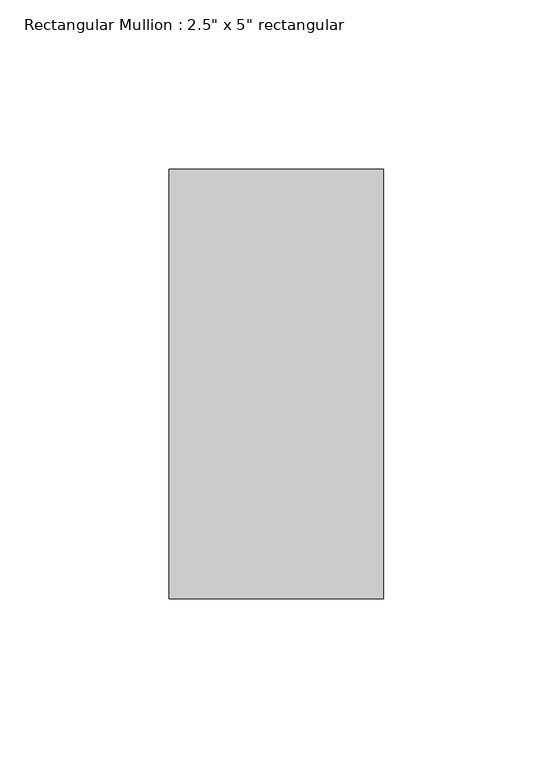
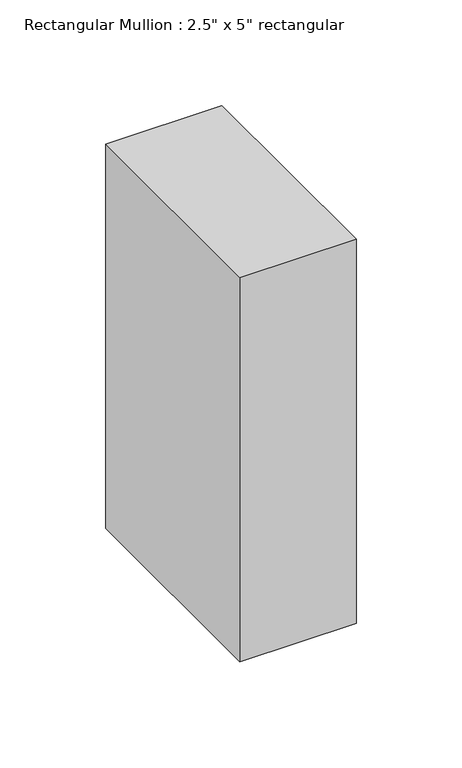
"""IFC4 building model written with IfcOpenShell, lengths in millimetres: member geometry."""

from ifc_helpers import new_model, si_unit, frame, origin, place, context, project, spatial, polyline, outline, extrude, source, transform, mapped, element, save


def member_d8da5bea(model_context):
    return source(origin(), model_context, "Body", "SweptSolid", [
        extrude(outline(polyline([(0.0, 63.5), (0.0, -63.5), (-63.5, -63.5), (-63.5, 63.5), (0.0, 63.5)])), frame((0.0, 0.0, -222.25), z_axis=(0.0, 0.0, 1.0), x_axis=(1.0, 0.0, 0.0)), (0.0, 0.0, 1.0), 222.25),
    ])


if __name__ == "__main__":
    model = new_model("IFC4")
    model_context = context("Model", 3, world=origin())
    ifc_project = project(units=[si_unit("LENGTHUNIT", "METRE", prefix="MILLI")], contexts=[model_context])
    site = spatial("IfcSite", under=ifc_project)
    building = spatial("IfcBuilding", under=site)
    placement = place(None, origin())
    member_shape = member_d8da5bea(model_context)
    element("IfcMember", 1, ObjectType="Rectangular Mullion : 2.5\" x 5\" rectangular", at=placement, inside=building, context=model_context, shape_type="MappedRepresentation", body=[
        mapped(member_shape, transform((0.0, 0.0, 0.0), x_axis=(1.0, 0.0, 0.0), y_axis=(0.0, 1.0, 0.0), z_axis=(0.0, 0.0, 1.0))),
    ])
    save(model, "model.ifc")

# Revit data of these elements
# Type "Rectangular Mullion : 2.5\" x 5\" rectangular"
#   built-in parameter 1007304 = 0.416667 (stored number, unit not read)
#   built-in parameter 1007301 = 0.104167 (stored number, unit not read)
#   built-in parameter 1007300 = 0.104167 (stored number, unit not read)
# Element 1 (IfcMember, "Rectangular Mullion : 2.5\" x 5\" rectangular")
#   Materials on its faces: "Aluminum"
# Materials
#   "Aluminum": class "Metal", colour RGB 247 247 247, transparency 0, Description = "Aluminum 6061", Cost = 0
